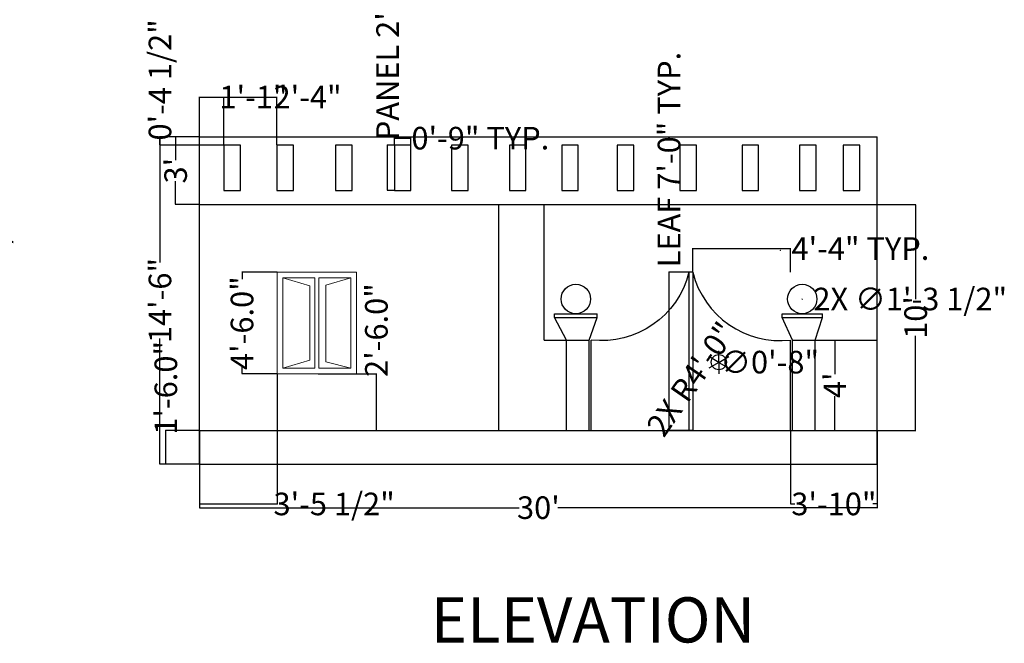
# Model space of a CAD drawing. Units: inches. Extents: x -91 to 1027, y -85 to 599.
# Tile 2 of 3: x 504 to 1027, y -84 to 248. Entities that reach past the tile are written whole.
import ezdxf

# ---------------------------------------------------------------- set-up
doc = ezdxf.new("R2010")
doc.units = ezdxf.units.IN
doc.header["$MEASUREMENT"] = 0
for name, color, linetype, lineweight in [('A-ANNO-DIMS', 2, 'Continuous', 18), ('A-ANNO-TEXT', 7, 'Continuous', 35), ('A-ELEV', 7, 'Continuous', 25), ('A-ELEV-GATE', 3, 'Continuous', 25), ('A-ELEV-GLAZ', 4, 'Continuous', 18), ('A-ELEV-PRPT', 7, 'Continuous', 25)]:
    doc.layers.add(name, color=color, linetype=linetype, lineweight=lineweight)
doc.styles.get("Standard").update_dxf_attribs({"font": 'arial.ttf'})
doc.dimstyles.get("Standard").update_dxf_attribs({"dimtxt": 12, "dimasz": 0.18, "dimexe": 0.18, "dimexo": 0.0625, "dimgap": 0.09, "dimtad": 0, "dimdec": 1, "dimzin": 0, "dimdsep": 46, "dimlunit": 3, "dimtxsty": 'Standard', "dimcen": 0.09, "dimadec": 0, "dimazin": 0, "dimtfac": 1, "dimtdec": 1, "dimtofl": 0, "dimtmove": 0, "dimatfit": 3, "dimfxl": 1, "dimtolj": 1, "dimtzin": 0, "dimarcsym": 0})

# ---------------------------------------------------------------- blocks, each defined once
blk = doc.blocks.new('*U3')
blk.add_line((0, 3.08), (0, -3.08))
blk = doc.blocks.new('*U4')
at = {"layer": 'A-ELEV-GATE', "color": 0, "linetype": 'ByBlock', "lineweight": -2, "transparency": 16777216}
for p, rotation in [((298.36, -261.46), 240), ((301.02, -259.92), 180), ((303.68, -261.46), 119.9999999999999), ((298.36, -264.53), 300), ((303.68, -264.53), 59.99999999999997)]:
    blk.add_blockref('*U3', p, dxfattribs=dict(at, rotation=rotation))
blk.add_blockref('*U3', (301.02, -266.07), dxfattribs=at)
blk = doc.blocks.new('*D9')
at = {"layer": 'A-ANNO-DIMS', "color": 0, "lineweight": -2, "transparency": 16777216}
for p, q in [((662.48, 59.43), (693.55, 59.43)), ((693.37, 59.43), (693.37, 59.61)), ((693.37, 29.61), (693.37, 59.25)), ((662.48, 29.43), (693.55, 29.43))]:
    blk.add_line(p, q, dxfattribs=at)
at = {"layer": 'A-ANNO-DIMS', "color": 0, "transparency": 16777216}
for points in [[(693.34, 59.25), (693.4, 59.25), (693.37, 59.43)], [(693.34, 29.61), (693.4, 29.61), (693.37, 29.43)]]:
    blk.add_solid(points, dxfattribs=at)
at = {"layer": 'Defpoints', "color": 0, "transparency": 16777216}
for p in [(662.42, 59.43), (693.37, 59.43), (662.42, 29.43)]:
    blk.add_point(p, dxfattribs=at)
at = {"layer": 'A-ANNO-DIMS', "color": 0, "transparency": 16777216, "insert": (693.37, 82.74), "char_height": 12, "attachment_point": 5, "rotation": 90}
blk.add_mtext('\\A1;2\'-6.0"', dxfattribs=at)
blk = doc.blocks.new('*D10')
at = {"layer": 'A-ANNO-DIMS', "color": 0, "lineweight": -2, "transparency": 16777216}
for p, q in [((640.68, 113.43), (621.81, 113.43)), ((621.99, 113.25), (621.99, 109.7)), ((621.99, 59.61), (621.99, 63.15)), ((640.68, 59.43), (621.81, 59.43))]:
    blk.add_line(p, q, dxfattribs=at)
at = {"layer": 'A-ANNO-DIMS', "color": 0, "transparency": 16777216}
for points in [[(621.96, 113.25), (622.02, 113.25), (621.99, 113.43)], [(621.96, 59.61), (622.02, 59.61), (621.99, 59.43)]]:
    blk.add_solid(points, dxfattribs=at)
at = {"layer": 'Defpoints', "color": 0, "transparency": 16777216}
for p in [(621.99, 113.43), (640.74, 113.43), (640.74, 59.43)]:
    blk.add_point(p, dxfattribs=at)
at = {"layer": 'A-ANNO-DIMS', "color": 0, "transparency": 16777216, "insert": (621.99, 86.43), "char_height": 12, "attachment_point": 5, "rotation": 90}
blk.add_mtext('\\A1;4\'-6.0"', dxfattribs=at)
blk = doc.blocks.new('*D11')
at = {"layer": 'A-ANNO-DIMS', "color": 0, "lineweight": -2, "transparency": 16777216}
for p, q in [((959.51, 149.43), (980.06, 149.43)), ((979.88, 149.25), (979.88, 99.13)), ((979.88, 29.61), (979.88, 79.72)), ((959.51, 29.43), (980.06, 29.43))]:
    blk.add_line(p, q, dxfattribs=at)
at = {"layer": 'A-ANNO-DIMS', "color": 0, "transparency": 16777216}
for points in [[(979.85, 149.25), (979.91, 149.25), (979.88, 149.43)], [(979.85, 29.61), (979.91, 29.61), (979.88, 29.43)]]:
    blk.add_solid(points, dxfattribs=at)
at = {"layer": 'Defpoints', "color": 0, "transparency": 16777216}
for p in [(959.45, 149.43), (979.88, 149.43), (959.45, 29.43)]:
    blk.add_point(p, dxfattribs=at)
at = {"layer": 'A-ANNO-DIMS', "color": 0, "transparency": 16777216, "insert": (979.88, 89.43), "char_height": 12, "attachment_point": 5, "rotation": 90}
blk.add_mtext("\\A1;10'", dxfattribs=at)
blk = doc.blocks.new('*D12')
at = {"layer": 'A-ANNO-DIMS', "color": 0, "lineweight": -2, "transparency": 16777216}
for p, q in [((599.45, 11.36), (599.45, -11.78)), ((959.45, 11.36), (959.45, -11.78)), ((599.63, -11.6), (769.18, -11.6)), ((959.27, -11.6), (789.72, -11.6))]:
    blk.add_line(p, q, dxfattribs=at)
at = {"layer": 'A-ANNO-DIMS', "color": 0, "transparency": 16777216}
for points in [[(599.63, -11.57), (599.63, -11.63), (599.45, -11.6)], [(959.27, -11.57), (959.27, -11.63), (959.45, -11.6)]]:
    blk.add_solid(points, dxfattribs=at)
at = {"layer": 'Defpoints', "color": 0, "transparency": 16777216}
for p in [(599.45, 11.43), (959.45, 11.43), (959.45, -11.6)]:
    blk.add_point(p, dxfattribs=at)
at = {"layer": 'A-ANNO-DIMS', "color": 0, "transparency": 16777216, "insert": (779.45, -11.6), "char_height": 12, "attachment_point": 5}
blk.add_mtext("\\A1;30'", dxfattribs=at)
blk = doc.blocks.new('*D13')
at = {"layer": 'A-ANNO-DIMS', "color": 0, "lineweight": -2, "transparency": 16777216}
for p, q in [((599.39, 29.43), (581.33, 29.43)), ((581.51, 29.43), (581.51, 29.61)), ((581.51, 11.61), (581.51, 29.25)), ((599.39, 11.43), (581.33, 11.43))]:
    blk.add_line(p, q, dxfattribs=at)
at = {"layer": 'A-ANNO-DIMS', "color": 0, "transparency": 16777216}
for points in [[(581.48, 29.25), (581.54, 29.25), (581.51, 29.43)], [(581.48, 11.61), (581.54, 11.61), (581.51, 11.43)]]:
    blk.add_solid(points, dxfattribs=at)
at = {"layer": 'Defpoints', "color": 0, "transparency": 16777216}
for p in [(581.51, 29.43), (599.45, 29.43), (599.45, 11.43)]:
    blk.add_point(p, dxfattribs=at)
at = {"layer": 'A-ANNO-DIMS', "color": 0, "transparency": 16777216, "insert": (581.51, 52.07), "char_height": 12, "attachment_point": 5, "rotation": 90}
blk.add_mtext('\\A1;1\'-6.0"', dxfattribs=at)
blk = doc.blocks.new('*D14')
at = {"layer": 'A-ANNO-DIMS', "color": 0, "lineweight": -2, "transparency": 16777216}
for p, q in [((926.51, 77.43), (937.13, 77.43)), ((936.95, 77.25), (936.95, 59.28)), ((936.95, 29.61), (936.95, 47.57)), ((926.51, 29.43), (937.13, 29.43))]:
    blk.add_line(p, q, dxfattribs=at)
at = {"layer": 'A-ANNO-DIMS', "color": 0, "transparency": 16777216}
for points in [[(936.92, 77.25), (936.98, 77.25), (936.95, 77.43)], [(936.92, 29.61), (936.98, 29.61), (936.95, 29.43)]]:
    blk.add_solid(points, dxfattribs=at)
at = {"layer": 'Defpoints', "color": 0, "transparency": 16777216}
for p in [(926.45, 77.43), (936.95, 77.43), (926.45, 29.43)]:
    blk.add_point(p, dxfattribs=at)
at = {"layer": 'A-ANNO-DIMS', "color": 0, "transparency": 16777216, "insert": (936.95, 53.43), "char_height": 12, "attachment_point": 5, "rotation": 90}
blk.add_mtext("\\A1;4'", dxfattribs=at)
blk = doc.blocks.new('*D15')
at = {"layer": 'A-ANNO-DIMS', "color": 0, "lineweight": -2, "transparency": 16777216}
for p, q in [((599.39, 185.43), (586.55, 185.43)), ((586.73, 185.25), (586.73, 173.03)), ((586.73, 149.61), (586.73, 161.82)), ((599.39, 149.43), (586.55, 149.43))]:
    blk.add_line(p, q, dxfattribs=at)
at = {"layer": 'A-ANNO-DIMS', "color": 0, "transparency": 16777216}
for points in [[(586.7, 185.25), (586.76, 185.25), (586.73, 185.43)], [(586.7, 149.61), (586.76, 149.61), (586.73, 149.43)]]:
    blk.add_solid(points, dxfattribs=at)
at = {"layer": 'Defpoints', "color": 0, "transparency": 16777216}
for p in [(586.73, 185.43), (599.45, 185.43), (599.45, 149.43)]:
    blk.add_point(p, dxfattribs=at)
at = {"layer": 'A-ANNO-DIMS', "color": 0, "transparency": 16777216, "insert": (586.73, 167.43), "char_height": 12, "attachment_point": 5, "rotation": 90}
blk.add_mtext("\\A1;3'", dxfattribs=at)
blk = doc.blocks.new('GATE-LEAF-ELEV')
for p, q in [((0, 84), (0, 0)), ((52, 0), (52, 48))]:
    blk.add_line(p, q)
blk.add_arc((46.55, 95.68), 47.99, 194.0856, 276.5241)
blk = doc.blocks.new('PARAPET-PANEL-ELEV')
blk.add_lwpolyline([(0, 0), (8.78, 0), (8.78, 24.23), (0, 24.23)], close=True)
blk = doc.blocks.new('GATE-POST-GLOBE')
blk.add_circle((7.81, 7.81), 7.81)
blk = doc.blocks.new('*D30')
at = {"layer": 'A-ANNO-DIMS', "color": 0, "lineweight": -2, "transparency": 16777216}
for p, q in [((702.92, 181.03), (699.16, 181.03)), ((699.34, 181.03), (699.34, 181.21)), ((699.34, 156.99), (699.34, 180.85)), ((702.92, 156.81), (699.16, 156.81))]:
    blk.add_line(p, q, dxfattribs=at)
at = {"layer": 'A-ANNO-DIMS', "color": 0, "transparency": 16777216}
for points in [[(699.31, 180.85), (699.37, 180.85), (699.34, 181.03)], [(699.31, 156.99), (699.37, 156.99), (699.34, 156.81)]]:
    blk.add_solid(points, dxfattribs=at)
at = {"layer": 'Defpoints', "color": 0, "transparency": 16777216}
for p in [(699.34, 181.03), (702.98, 181.03), (702.98, 156.81)]:
    blk.add_point(p, dxfattribs=at)
at = {"layer": 'A-ANNO-DIMS', "color": 0, "transparency": 16777216, "insert": (699.34, 247.39), "char_height": 12, "attachment_point": 5, "rotation": 90}
blk.add_mtext('\\A1;PANEL 2\'-0" TYP.', dxfattribs=at)
blk = doc.blocks.new('*D31')
at = {"layer": 'A-ANNO-DIMS', "color": 0, "lineweight": -2, "transparency": 16777216}
for p, q in [((702.98, 181.1), (702.98, 184.85)), ((703.16, 184.67), (711.58, 184.67)), ((711.76, 181.1), (711.76, 184.85)), ((711.76, 184.67), (711.94, 184.67))]:
    blk.add_line(p, q, dxfattribs=at)
at = {"layer": 'A-ANNO-DIMS', "color": 0, "transparency": 16777216}
for points in [[(703.16, 184.7), (703.16, 184.64), (702.98, 184.67)], [(711.58, 184.7), (711.58, 184.64), (711.76, 184.67)]]:
    blk.add_solid(points, dxfattribs=at)
at = {"layer": 'Defpoints', "color": 0, "transparency": 16777216}
for p in [(711.76, 184.67), (702.98, 181.03), (711.76, 181.03)]:
    blk.add_point(p, dxfattribs=at)
at = {"layer": 'A-ANNO-DIMS', "color": 0, "transparency": 16777216, "insert": (748.61, 184.67), "char_height": 12, "attachment_point": 5}
blk.add_mtext('\\A1;0\'-9" TYP.', dxfattribs=at)
blk = doc.blocks.new('*D34')
at = {"layer": 'A-ANNO-DIMS', "color": 0, "lineweight": -2, "transparency": 16777216}
for p, q in [((861.39, 113.43), (848.67, 113.43)), ((848.85, 113.43), (848.85, 113.61)), ((848.85, 29.61), (848.85, 113.25)), ((861.39, 29.43), (848.67, 29.43))]:
    blk.add_line(p, q, dxfattribs=at)
at = {"layer": 'A-ANNO-DIMS', "color": 0, "transparency": 16777216}
for points in [[(848.82, 113.25), (848.88, 113.25), (848.85, 113.43)], [(848.82, 29.61), (848.88, 29.61), (848.85, 29.43)]]:
    blk.add_solid(points, dxfattribs=at)
at = {"layer": 'Defpoints', "color": 0, "transparency": 16777216}
for p in [(848.85, 113.43), (861.45, 113.43), (861.45, 29.43)]:
    blk.add_point(p, dxfattribs=at)
at = {"layer": 'A-ANNO-DIMS', "color": 0, "transparency": 16777216, "insert": (848.85, 173.3), "char_height": 12, "attachment_point": 5, "rotation": 90}
blk.add_mtext('\\A1;LEAF 7\'-0" TYP.', dxfattribs=at)
blk = doc.blocks.new('*D35')
at = {"layer": 'A-ANNO-DIMS', "color": 0, "lineweight": -2, "transparency": 16777216}
for p, q in [((861.45, 113.49), (861.45, 126.21)), ((861.63, 126.03), (913.27, 126.03)), ((913.45, 113.49), (913.45, 126.21)), ((913.45, 126.03), (913.63, 126.03))]:
    blk.add_line(p, q, dxfattribs=at)
at = {"layer": 'A-ANNO-DIMS', "color": 0, "transparency": 16777216}
for points in [[(861.63, 126.06), (861.63, 126), (861.45, 126.03)], [(913.27, 126.06), (913.27, 126), (913.45, 126.03)]]:
    blk.add_solid(points, dxfattribs=at)
at = {"layer": 'Defpoints', "color": 0, "transparency": 16777216}
for p in [(913.45, 126.03), (861.45, 113.43), (913.45, 113.43)]:
    blk.add_point(p, dxfattribs=at)
at = {"layer": 'A-ANNO-DIMS', "color": 0, "transparency": 16777216, "insert": (950.54, 126.03), "char_height": 12, "attachment_point": 5}
blk.add_mtext('\\A1;4\'-4" TYP.', dxfattribs=at)
blk = doc.blocks.new('*D45')
at = {"layer": 'A-ANNO-DIMS', "color": 0, "lineweight": -2, "transparency": 16777216}
for p, q in [((385.21, 225.81), (491.83, 225.81)), ((491.65, 225.63), (491.65, 149.28)), ((491.65, 4.7), (491.65, 81.05)), ((385.21, 4.52), (491.83, 4.52))]:
    blk.add_line(p, q, dxfattribs=at)
at = {"layer": 'A-ANNO-DIMS', "color": 0, "transparency": 16777216}
for points in [[(491.62, 225.63), (491.68, 225.63), (491.65, 225.81)], [(491.62, 4.7), (491.68, 4.7), (491.65, 4.52)]]:
    blk.add_solid(points, dxfattribs=at)
at = {"layer": 'Defpoints', "color": 0, "transparency": 16777216}
for p in [(385.15, 225.81), (491.65, 225.81), (385.15, 4.52)]:
    blk.add_point(p, dxfattribs=at)
at = {"layer": 'A-ANNO-DIMS', "color": 0, "transparency": 16777216, "insert": (491.65, 115.17), "char_height": 12, "attachment_point": 5, "rotation": 90}
blk.add_mtext('\\A1;18\'-5 1/2"', dxfattribs=at)
blk = doc.blocks.new('*D62')
at = {"layer": 'A-ANNO-DIMS', "color": 0, "lineweight": -2, "transparency": 16777216}
for p, q in [((599.39, 185.43), (578.22, 185.43)), ((578.4, 185.25), (578.4, 118.56)), ((578.4, 11.61), (578.4, 78.29)), ((599.39, 11.43), (578.22, 11.43))]:
    blk.add_line(p, q, dxfattribs=at)
at = {"layer": 'A-ANNO-DIMS', "color": 0, "transparency": 16777216}
for points in [[(578.37, 185.25), (578.43, 185.25), (578.4, 185.43)], [(578.37, 11.61), (578.43, 11.61), (578.4, 11.43)]]:
    blk.add_solid(points, dxfattribs=at)
at = {"layer": 'Defpoints', "color": 0, "transparency": 16777216}
for p in [(578.4, 185.43), (599.45, 185.43), (599.45, 11.43)]:
    blk.add_point(p, dxfattribs=at)
at = {"layer": 'A-ANNO-DIMS', "color": 0, "transparency": 16777216, "insert": (578.4, 98.43), "char_height": 12, "attachment_point": 5, "rotation": 90}
blk.add_mtext('\\A1;14\'-6"', dxfattribs=at)
blk = doc.blocks.new('*D63')
at = {"layer": 'A-ANNO-DIMS', "color": 0, "lineweight": -2, "transparency": 16777216}
for p, q in [((640.74, 59.36), (640.74, -9.8)), ((599.45, 29.36), (599.45, -9.8)), ((599.63, -9.62), (640.56, -9.62)), ((640.74, -9.62), (640.92, -9.62))]:
    blk.add_line(p, q, dxfattribs=at)
at = {"layer": 'A-ANNO-DIMS', "color": 0, "transparency": 16777216}
for points in [[(599.63, -9.59), (599.63, -9.65), (599.45, -9.62)], [(640.56, -9.59), (640.56, -9.65), (640.74, -9.62)]]:
    blk.add_solid(points, dxfattribs=at)
at = {"layer": 'Defpoints', "color": 0, "transparency": 16777216}
for p in [(640.74, 59.43), (599.45, 29.43), (640.74, -9.62)]:
    blk.add_point(p, dxfattribs=at)
at = {"layer": 'A-ANNO-DIMS', "color": 0, "transparency": 16777216, "insert": (670.94, -9.62), "char_height": 12, "attachment_point": 5}
blk.add_mtext('\\A1;3\'-5 1/2"', dxfattribs=at)
blk = doc.blocks.new('*D64')
at = {"layer": 'A-ANNO-DIMS', "color": 0, "lineweight": -2, "transparency": 16777216}
for p, q in [((599.45, 185.49), (599.45, 206.66)), ((599.63, 206.48), (612.23, 206.48)), ((612.41, 181.1), (612.41, 206.66)), ((612.41, 206.48), (612.59, 206.48))]:
    blk.add_line(p, q, dxfattribs=at)
at = {"layer": 'A-ANNO-DIMS', "color": 0, "transparency": 16777216}
for points in [[(599.63, 206.51), (599.63, 206.45), (599.45, 206.48)], [(612.23, 206.51), (612.23, 206.45), (612.41, 206.48)]]:
    blk.add_solid(points, dxfattribs=at)
at = {"layer": 'Defpoints', "color": 0, "transparency": 16777216}
for p in [(612.41, 206.48), (599.45, 185.43), (612.41, 181.03)]:
    blk.add_point(p, dxfattribs=at)
at = {"layer": 'A-ANNO-DIMS', "color": 0, "transparency": 16777216, "insert": (628.07, 206.48), "char_height": 12, "attachment_point": 5}
blk.add_mtext('\\A1;1\'-1"', dxfattribs=at)
blk = doc.blocks.new('*D65')
at = {"layer": 'A-ANNO-DIMS', "color": 0, "lineweight": -2, "transparency": 16777216}
for p, q in [((612.41, 181.1), (612.41, 206.66)), ((612.59, 206.48), (640.33, 206.48)), ((640.51, 181.1), (640.51, 206.66)), ((640.51, 206.48), (640.69, 206.48))]:
    blk.add_line(p, q, dxfattribs=at)
at = {"layer": 'A-ANNO-DIMS', "color": 0, "transparency": 16777216}
for points in [[(612.59, 206.51), (612.59, 206.45), (612.41, 206.48)], [(640.33, 206.51), (640.33, 206.45), (640.51, 206.48)]]:
    blk.add_solid(points, dxfattribs=at)
at = {"layer": 'Defpoints', "color": 0, "transparency": 16777216}
for p in [(640.51, 206.48), (612.41, 181.03), (640.51, 181.03)]:
    blk.add_point(p, dxfattribs=at)
at = {"layer": 'A-ANNO-DIMS', "color": 0, "transparency": 16777216, "insert": (656.83, 206.48), "char_height": 12, "attachment_point": 5}
blk.add_mtext('\\A1;2\'-4"', dxfattribs=at)
blk = doc.blocks.new('*D66')
at = {"layer": 'A-ANNO-DIMS', "color": 0, "lineweight": -2, "transparency": 16777216}
for p, q in [((599.39, 185.43), (578.22, 185.43)), ((578.4, 185.43), (578.4, 185.61)), ((578.4, 181.21), (578.4, 185.25)), ((612.35, 181.03), (578.22, 181.03))]:
    blk.add_line(p, q, dxfattribs=at)
at = {"layer": 'A-ANNO-DIMS', "color": 0, "transparency": 16777216}
for points in [[(578.37, 185.25), (578.43, 185.25), (578.4, 185.43)], [(578.37, 181.21), (578.43, 181.21), (578.4, 181.03)]]:
    blk.add_solid(points, dxfattribs=at)
at = {"layer": 'Defpoints', "color": 0, "transparency": 16777216}
for p in [(578.4, 185.43), (599.45, 185.43), (612.41, 181.03)]:
    blk.add_point(p, dxfattribs=at)
at = {"layer": 'A-ANNO-DIMS', "color": 0, "transparency": 16777216, "insert": (578.4, 215.63), "char_height": 12, "attachment_point": 5, "rotation": 90}
blk.add_mtext('\\A1;0\'-4 1/2"', dxfattribs=at)
blk = doc.blocks.new('*D67')
at = {"layer": 'A-ANNO-DIMS', "color": 0, "lineweight": -2, "transparency": 16777216}
for p, q in [((913.45, 29.36), (913.45, -9.8)), ((959.45, 29.36), (959.45, -9.8)), ((913.63, -9.62), (915.75, -9.62)), ((959.27, -9.62), (957.15, -9.62))]:
    blk.add_line(p, q, dxfattribs=at)
at = {"layer": 'A-ANNO-DIMS', "color": 0, "transparency": 16777216}
for points in [[(913.63, -9.59), (913.63, -9.65), (913.45, -9.62)], [(959.27, -9.59), (959.27, -9.65), (959.45, -9.62)]]:
    blk.add_solid(points, dxfattribs=at)
at = {"layer": 'Defpoints', "color": 0, "transparency": 16777216}
for p in [(913.45, 29.43), (959.45, 29.43), (913.45, -9.62)]:
    blk.add_point(p, dxfattribs=at)
at = {"layer": 'A-ANNO-DIMS', "color": 0, "transparency": 16777216, "insert": (936.45, -9.62), "char_height": 12, "attachment_point": 5}
blk.add_mtext('\\A1;3\'-10"', dxfattribs=at)
blk = doc.blocks.new('*D70')
at = {"layer": 'A-ANNO-DIMS', "color": 0, "lineweight": -2, "transparency": 16777216}
for p, q in [((907.91, 125.11), (908.09, 125.11)), ((908, 125.02), (908, 125.2)), ((880.48, 85.35), (880.58, 85.5))]:
    blk.add_line(p, q, dxfattribs=at)
at = {"layer": 'A-ANNO-DIMS', "color": 0, "transparency": 16777216}
blk.add_solid([(880.55, 85.52), (880.6, 85.48), (880.68, 85.65)], dxfattribs=at)
at = {"layer": 'Defpoints', "color": 0, "transparency": 16777216}
for p in [(908, 125.11), (880.68, 85.65)]:
    blk.add_point(p, dxfattribs=at)
at = {"layer": 'A-ANNO-DIMS', "color": 0, "transparency": 16777216, "insert": (860.68, 56.76), "char_height": 12, "attachment_point": 5, "rotation": 55.3048}
blk.add_mtext('\\A1;2X R4\'-0"', dxfattribs=at)
blk = doc.blocks.new('*D71')
at = {"layer": 'A-ANNO-DIMS', "color": 0, "lineweight": -2, "transparency": 16777216}
for p, q in [((919.54, 99.23), (919.72, 99.23)), ((919.63, 99.14), (919.63, 99.32)), ((927.79, 99.23), (927.61, 99.23))]:
    blk.add_line(p, q, dxfattribs=at)
at = {"layer": 'A-ANNO-DIMS', "color": 0, "transparency": 16777216}
blk.add_solid([(927.61, 99.26), (927.61, 99.2), (927.43, 99.23)], dxfattribs=at)
at = {"layer": 'Defpoints', "color": 0, "transparency": 16777216}
for p in [(911.82, 99.23), (927.43, 99.23)]:
    blk.add_point(p, dxfattribs=at)
at = {"layer": 'A-ANNO-DIMS', "color": 0, "transparency": 16777216, "insert": (977.02, 99.23), "char_height": 12, "attachment_point": 5, "rotation": 359.9986}
blk.add_mtext('\\A1;2X ∅1\'-3 1/2"', dxfattribs=at)
blk = doc.blocks.new('*D72')
at = {"layer": 'A-ANNO-DIMS', "color": 0, "lineweight": -2, "transparency": 16777216}
for p, q in [((875.24, 65.7), (875.42, 65.7)), ((875.33, 65.61), (875.33, 65.79)), ((879.73, 65.7), (879.55, 65.7))]:
    blk.add_line(p, q, dxfattribs=at)
at = {"layer": 'A-ANNO-DIMS', "color": 0, "transparency": 16777216}
blk.add_solid([(879.55, 65.73), (879.55, 65.67), (879.37, 65.7)], dxfattribs=at)
at = {"layer": 'Defpoints', "color": 0, "transparency": 16777216}
for p in [(871.28, 65.7), (879.37, 65.7)]:
    blk.add_point(p, dxfattribs=at)
at = {"layer": 'A-ANNO-DIMS', "color": 0, "transparency": 16777216, "insert": (902.3, 65.7), "char_height": 12, "attachment_point": 5, "rotation": 359.9949}
blk.add_mtext('\\A1;∅0\'-8"', dxfattribs=at)

msp = doc.modelspace()

# ---------------------------------------------------------------- linework, layer by layer
at = {"layer": 'A-ELEV'}
for p, q in [((599.45, 11.43), (599.45, 185.43)), ((959.45, 11.43), (959.45, 185.43)), ((758.45, 29.43), (758.45, 149.43)), ((782.45, 77.43), (782.45, 149.43)), ((599.45, 29.43), (959.45, 29.43)), ((599.45, 11.43), (959.45, 11.43))]:
    msp.add_line(p, q, dxfattribs=at)
at = {"layer": 'A-ELEV-GATE'}
for p, q in [((788.07, 91.43), (810.67, 91.43)), ((788.07, 89.43), (788.07, 91.43)), ((788.07, 89.43), (810.67, 89.43)), ((794.45, 77.43), (788.07, 89.43)), ((806.45, 77.43), (810.67, 89.43)), ((810.67, 89.43), (810.67, 91.43)), ((908.9, 91.43), (930.34, 91.43)), ((908.9, 89.43), (908.9, 91.43)), ((908.9, 89.43), (930.34, 89.43)), ((914.45, 77.43), (908.9, 89.43)), ((926.45, 77.43), (930.34, 89.43)), ((930.34, 89.43), (930.34, 91.43)), ((782.45, 77.43), (806.45, 77.43)), ((794.45, 29.43), (794.45, 77.43)), ((806.45, 29.43), (806.45, 77.43)), ((914.45, 29.43), (914.45, 77.43)), ((914.45, 77.43), (959.45, 77.43)), ((926.45, 29.43), (926.45, 77.43))]:
    msp.add_line(p, q, dxfattribs=at)
msp.add_circle((875.33, 65.7), 4.05, dxfattribs=at)
at = {"layer": 'A-ELEV-GLAZ'}
for p, q in [((643.74, 110.43), (660.74, 110.43)), ((643.74, 62.43), (643.74, 110.43)), ((643.74, 110.43), (658.05, 106.21)), ((660.74, 62.43), (660.74, 110.43)), ((662.74, 62.43), (662.74, 110.43)), ((662.74, 110.43), (679.74, 110.43)), ((679.74, 110.43), (666.47, 106.6)), ((679.74, 110.43), (679.74, 62.43)), ((658.05, 106.21), (658.05, 66.73)), ((666.47, 106.6), (666.47, 65.87)), ((658.05, 66.73), (643.74, 62.43)), ((666.47, 65.87), (679.74, 62.43)), ((660.74, 62.43), (643.74, 62.43)), ((679.74, 62.43), (662.74, 62.43))]:
    msp.add_line(p, q, dxfattribs=at)
msp.add_lwpolyline([(640.74, 113.43), (682.74, 113.43), (682.74, 59.43), (640.74, 59.43)], close=True, dxfattribs=at)
at = {"layer": 'A-ELEV-PRPT'}
for p, q in [((599.45, 185.43), (959.45, 185.43)), ((599.45, 149.43), (959.45, 149.43))]:
    msp.add_line(p, q, dxfattribs=at)

# ---------------------------------------------------------------- block references
at = {"layer": 'A-ELEV-GATE', "extrusion": (0, 0, -1), "zscale": -1}
msp.add_blockref('GATE-LEAF-ELEV', (-859.45, 29.43), dxfattribs=at)
at = {"layer": 'A-ELEV-GATE'}
for name, p in [('GATE-LEAF-ELEV', (861.45, 29.43)), ('GATE-POST-GLOBE', (791.55, 91.43)), ('GATE-POST-GLOBE', (911.82, 91.43)), ('*U4', (574.31, 328.57))]:
    msp.add_blockref(name, p, dxfattribs=at)
at = {"layer": 'A-ELEV-PRPT'}
for p in [(612.41, 156.81), (640.51, 156.81), (671.67, 156.81), (702.98, 156.81), (733.3, 156.81), (764.04, 156.81), (791.87, 156.81), (821.35, 156.81), (854.61, 156.81), (887.66, 156.81), (918.18, 156.81), (941.44, 156.81)]:
    msp.add_blockref('PARAPET-PANEL-ELEV', p, dxfattribs=at)

# ---------------------------------------------------------------- texts
at = {"layer": 'A-ANNO-TEXT'}
msp.add_text('ELEVATION', height=24, dxfattribs=at).set_placement((722.32, -83.22))

# ---------------------------------------------------------------- dimensions: what is measured, and where the dimension line sits
at = {"layer": 'A-ANNO-DIMS'}
for base, p1, p2, text, picture, middle in [((699.34, 181.03), (702.98, 156.81), (702.98, 181.03), 'PANEL <> TYP.', '*D30', (699.34, 247.39)), ((848.85, 113.43), (861.45, 29.43), (861.45, 113.43), 'LEAF <> TYP.', '*D34', (848.85, 173.3))]:
    dim = msp.add_linear_dim(base=base, p1=p1, p2=p2, angle=90, text=text, dimstyle='Standard', override={"dimdec": 1, "dimlfac": 1, "dimrnd": 0, "dimzin": 1, "dimdsep": 46, "dimlunit": 4, "dimfrac": 2}, dxfattribs=at)
    dim.commit()
    dim.dimension.update_dxf_attribs({"geometry": picture, "text_midpoint": middle})
for base, p1, p2, override, picture, middle in [((578.4, 185.43), (612.41, 181.03), (599.45, 185.43), {"dimdec": 1, "dimlfac": 1, "dimrnd": 0, "dimzin": 1, "dimdsep": 46, "dimlunit": 4, "dimfrac": 2}, '*D66', (578.4, 215.63)), ((491.65, 225.81), (385.15, 4.52), (385.15, 225.81), {"dimdec": 1, "dimlfac": 1, "dimrnd": 0, "dimzin": 1, "dimdsep": 46, "dimlunit": 4, "dimfrac": 2}, '*D45', (491.65, 115.17)), ((578.4, 185.43), (599.45, 11.43), (599.45, 185.43), {"dimdec": 1, "dimlfac": 1, "dimrnd": 0, "dimzin": 1, "dimdsep": 46, "dimlunit": 4, "dimfrac": 2}, '*D62', (578.4, 98.43)), ((586.73, 185.43), (599.45, 149.43), (599.45, 185.43), {"dimclrd": 0, "dimclre": 0, "dimclrt": 0}, '*D15', (586.73, 167.43)), ((979.88, 149.43), (959.45, 29.43), (959.45, 149.43), {"dimclrd": 0, "dimclre": 0, "dimclrt": 0}, '*D11', (979.88, 89.43)), ((621.99, 113.43), (640.74, 59.43), (640.74, 113.43), {"dimclrd": 0, "dimclre": 0, "dimclrt": 0}, '*D10', (621.99, 86.43)), ((693.37, 59.43), (662.42, 29.43), (662.42, 59.43), {"dimclrd": 0, "dimclre": 0, "dimclrt": 0}, '*D9', (693.37, 82.74)), ((581.51, 29.43), (599.45, 11.43), (599.45, 29.43), {"dimclrd": 0, "dimclre": 0, "dimclrt": 0}, '*D13', (581.51, 52.07)), ((936.95, 77.43), (926.45, 29.43), (926.45, 77.43), {"dimclrd": 0, "dimclre": 0, "dimclrt": 0}, '*D14', (936.95, 53.43))]:
    dim = msp.add_linear_dim(base=base, p1=p1, p2=p2, angle=90, dimstyle='Standard', override=override, dxfattribs=at)
    dim.commit()
    dim.dimension.update_dxf_attribs({"geometry": picture, "text_midpoint": middle})
for base, p1, p2, override, picture, middle in [((612.41, 206.48), (599.45, 185.43), (612.41, 181.03), {"dimdec": 1, "dimlfac": 1, "dimrnd": 0, "dimzin": 1, "dimdsep": 46, "dimlunit": 4, "dimfrac": 2}, '*D64', (628.07, 206.48)), ((640.51, 206.48), (612.41, 181.03), (640.51, 181.03), {"dimdec": 1, "dimlfac": 1, "dimrnd": 0, "dimzin": 1, "dimdsep": 46, "dimlunit": 4, "dimfrac": 2}, '*D65', (656.83, 206.48)), ((640.74, -9.62), (599.45, 29.43), (640.74, 59.43), {"dimdec": 1, "dimlfac": 1, "dimrnd": 0, "dimzin": 1, "dimdsep": 46, "dimlunit": 4, "dimfrac": 2}, '*D63', (670.94, -9.62)), ((913.45, -9.62), (959.45, 29.43), (913.45, 29.43), {"dimdec": 1, "dimlfac": 1, "dimrnd": 0, "dimzin": 1, "dimdsep": 46, "dimlunit": 4, "dimfrac": 2}, '*D67', (936.45, -9.62)), ((959.45, -11.6), (599.45, 11.43), (959.45, 11.43), {"dimclrd": 0, "dimclre": 0, "dimclrt": 0}, '*D12', (779.45, -11.6))]:
    dim = msp.add_linear_dim(base=base, p1=p1, p2=p2, dimstyle='Standard', override=override, dxfattribs=at)
    dim.commit()
    dim.dimension.update_dxf_attribs({"geometry": picture, "text_midpoint": middle})
for base, p1, p2, picture, middle in [((711.76, 184.67), (702.98, 181.03), (711.76, 181.03), '*D31', (748.61, 184.67)), ((913.45, 126.03), (861.45, 113.43), (913.45, 113.43), '*D35', (950.54, 126.03))]:
    dim = msp.add_linear_dim(base=base, p1=p1, p2=p2, text='<> TYP.', dimstyle='Standard', override={"dimdec": 1, "dimlfac": 1, "dimrnd": 0, "dimzin": 1, "dimdsep": 46, "dimlunit": 4, "dimfrac": 2}, dxfattribs=at)
    dim.commit()
    dim.dimension.update_dxf_attribs({"geometry": picture, "text_midpoint": middle})
dim = msp.add_diameter_dim_2p(p1=(911.82, 99.23), p2=(927.43, 99.23), text='2X <>', dimstyle='Standard', override={"dimdec": 1, "dimlfac": 1, "dimrnd": 0, "dimzin": 1, "dimdsep": 46, "dimlunit": 4, "dimfrac": 2}, dxfattribs=at)
dim.commit()
dim.dimension.update_dxf_attribs({"geometry": '*D71', "text_midpoint": (977.02, 99.23)})
dim = msp.add_radius_dim(center=(908, 125.11), mpoint=(880.68, 85.65), text='2X <>', dimstyle='Standard', override={"dimdec": 1, "dimlfac": 1, "dimrnd": 0, "dimzin": 1, "dimdsep": 46, "dimlunit": 4, "dimfrac": 2}, dxfattribs=at)
dim.commit()
dim.dimension.update_dxf_attribs({"geometry": '*D70', "text_midpoint": (860.68, 56.76)})
dim = msp.add_diameter_dim_2p(p1=(871.28, 65.7), p2=(879.37, 65.7), dimstyle='Standard', override={"dimdec": 1, "dimlfac": 1, "dimrnd": 0, "dimzin": 1, "dimdsep": 46, "dimlunit": 4, "dimfrac": 2}, dxfattribs=at)
dim.commit()
dim.dimension.update_dxf_attribs({"geometry": '*D72', "text_midpoint": (902.3, 65.7)})

doc.saveas('drawing.dxf')
